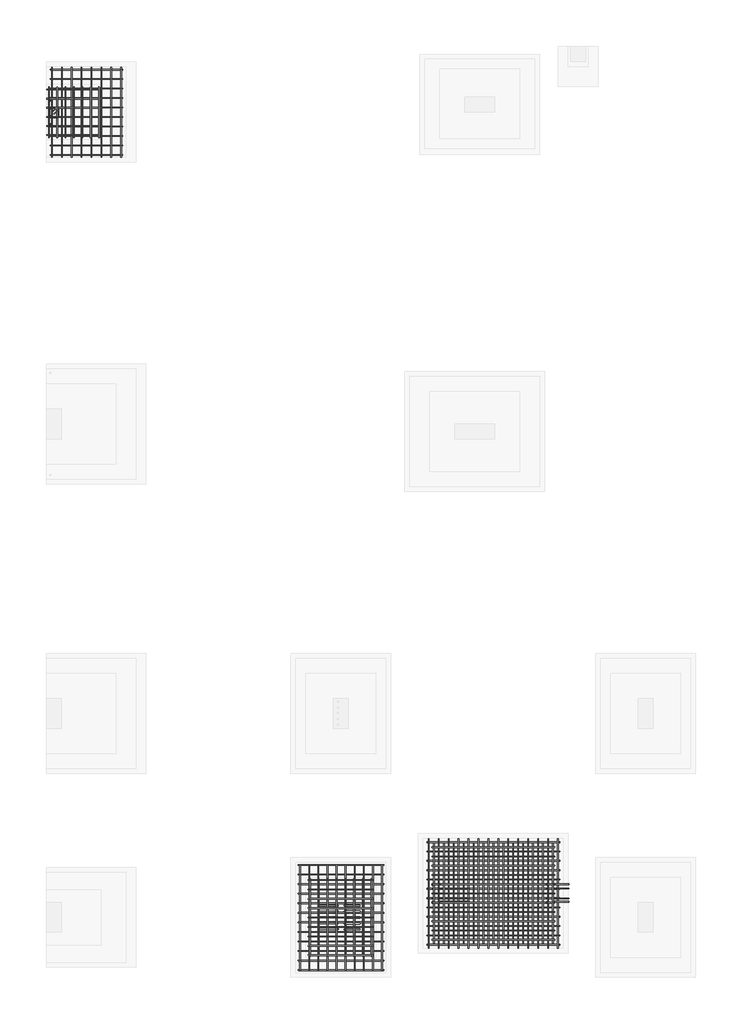
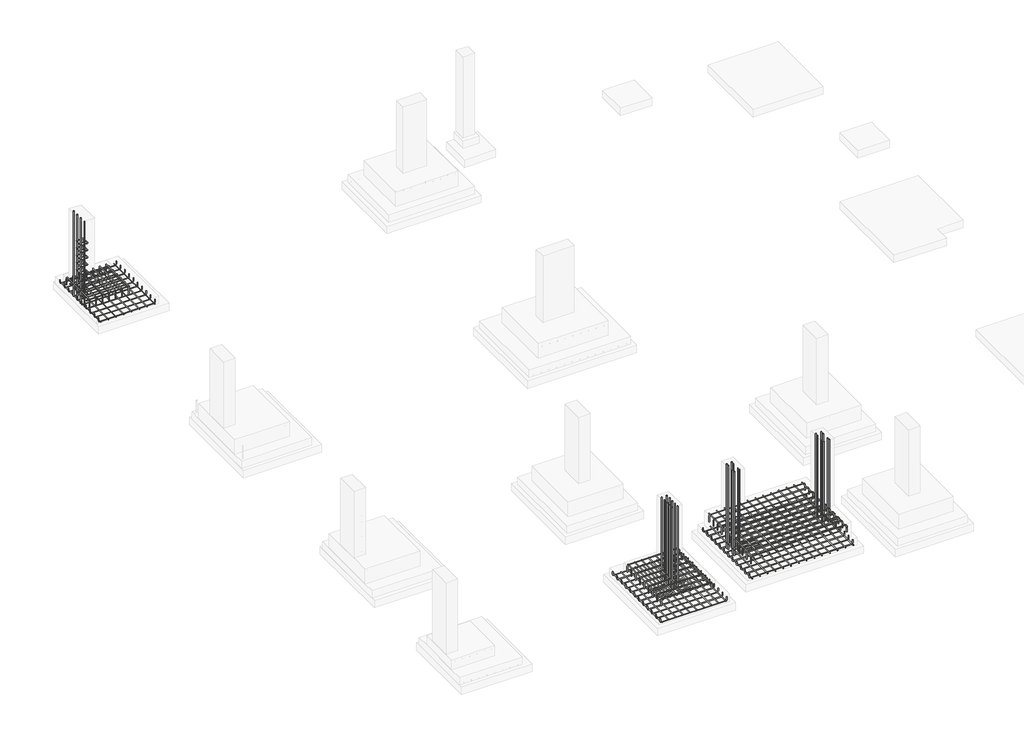
# One storey, part 3 of 6: 24 reinforcing bars.
"""IFC4 building model written with IfcOpenShell, lengths in millimetres."""

from ifc_helpers import new_model, si_unit, point, frame, origin, place, context, project, spatial, polyline, circle_curve, trimmed, segment, composite_curve, source, transform, mapped, element, save
from ifc_brep_helpers import swept_disk

model = new_model("IFC4")

# Units and contexts
model_context = context("Model", 3, world=origin())
ifc_project = project(units=[si_unit("LENGTHUNIT", "METRE", prefix="MILLI")], contexts=[model_context])

# Site, building, storey
site = spatial("IfcSite", under=ifc_project)
building = spatial("IfcBuilding", under=site)
storey = spatial("IfcBuildingStorey", under=building, Elevation=-1828.8)

# Reinforcing bars
placement = place(None, origin())
reinforcing_bar_shape = source(origin(), model_context, "Body", "SolidModel", [
    swept_disk(composite_curve([segment(polyline([(5667705.257242, -3596967.8875145, -1798.9561208), (5667705.257242, -3598584.2875145, -1798.9561208)]), True, "CONTINUOUS")], self_intersect=False), 6.0),
])
element("IfcReinforcingBar", 1, at=placement, inside=storey, context=model_context, shape_type="MappedRepresentation", body=[
    mapped(reinforcing_bar_shape, transform((0.0, 0.0, 0.0), x_axis=(1.0, 0.0, 0.0), y_axis=(0.0, 1.0, 0.0), z_axis=(0.0, 0.0, 1.0))),
    mapped(reinforcing_bar_shape, transform((-138.8763652, 0.0, 0.0), x_axis=(1.0, 0.0, 0.0), y_axis=(0.0, 1.0, 0.0), z_axis=(0.0, 0.0, 1.0))),
    mapped(reinforcing_bar_shape, transform((-277.7527305, 0.0, 0.0), x_axis=(1.0, 0.0, 0.0), y_axis=(0.0, 1.0, 0.0), z_axis=(0.0, 0.0, 1.0))),
    mapped(reinforcing_bar_shape, transform((-416.6290957, 0.0, 0.0), x_axis=(1.0, 0.0, 0.0), y_axis=(0.0, 1.0, 0.0), z_axis=(0.0, 0.0, 1.0))),
    mapped(reinforcing_bar_shape, transform((-555.5054609, 0.0, 0.0), x_axis=(1.0, 0.0, 0.0), y_axis=(0.0, 1.0, 0.0), z_axis=(0.0, 0.0, 1.0))),
    mapped(reinforcing_bar_shape, transform((-694.3818262, 0.0, 0.0), x_axis=(1.0, 0.0, 0.0), y_axis=(0.0, 1.0, 0.0), z_axis=(0.0, 0.0, 1.0))),
    mapped(reinforcing_bar_shape, transform((-833.2581914, 0.0, 0.0), x_axis=(1.0, 0.0, 0.0), y_axis=(0.0, 1.0, 0.0), z_axis=(0.0, 0.0, 1.0))),
    mapped(reinforcing_bar_shape, transform((-972.1345566, 0.0, 0.0), x_axis=(1.0, 0.0, 0.0), y_axis=(0.0, 1.0, 0.0), z_axis=(0.0, 0.0, 1.0))),
    mapped(reinforcing_bar_shape, transform((-1111.0109219, 0.0, 0.0), x_axis=(1.0, 0.0, 0.0), y_axis=(0.0, 1.0, 0.0), z_axis=(0.0, 0.0, 1.0))),
    mapped(reinforcing_bar_shape, transform((-1249.8872871, 0.0, 0.0), x_axis=(1.0, 0.0, 0.0), y_axis=(0.0, 1.0, 0.0), z_axis=(0.0, 0.0, 1.0))),
])
reinforcing_bar_2_shape = source(origin(), model_context, "Body", "SolidModel", [
    swept_disk(composite_curve([segment(polyline([(5666582.9165246, -3598349.6875145, -1653.2), (5666582.9165246, -3598349.6875145, -1539.2)]), True, "CONTINUOUS"), segment(trimmed(circle_curve(frame((5666612.9165246, -3598349.6875145, -1539.2), z_axis=(0.0, 1.0, 0.0), x_axis=(-30.0, 0.0, 0.0)), 30.0), [point((5666582.9165246, -3598349.6875145, -1539.2))], [point((5666612.9165246, -3598349.6875145, -1509.2))], True, "CARTESIAN"), True, "CONTINUOUS"), segment(polyline([(5666612.9165246, -3598349.6875145, -1509.2), (5667539.8524241, -3598349.6875145, -1509.2)]), True, "CONTINUOUS"), segment(trimmed(circle_curve(frame((5667539.8524241, -3598349.6875145, -1539.2), z_axis=(0.0, 1.0, 0.0), x_axis=(0.0, 0.0, 30.0)), 30.0), [point((5667539.8524241, -3598349.6875145, -1509.2))], [point((5667569.8524241, -3598349.6875145, -1539.2))], True, "CARTESIAN"), True, "CONTINUOUS"), segment(polyline([(5667569.8524241, -3598349.6875145, -1539.2), (5667569.8524241, -3598349.6875145, -1653.2)]), True, "CONTINUOUS")], self_intersect=False), 6.0),
])
element("IfcReinforcingBar", 2, at=placement, inside=storey, context=model_context, shape_type="MappedRepresentation", body=[
    mapped(reinforcing_bar_2_shape, transform((0.0, 0.0, 0.0), x_axis=(1.0, 0.0, 0.0), y_axis=(0.0, 1.0, 0.0), z_axis=(0.0, 0.0, 1.0))),
    mapped(reinforcing_bar_2_shape, transform((0.0, 143.4, 0.0), x_axis=(1.0, 0.0, 0.0), y_axis=(0.0, 1.0, 0.0), z_axis=(0.0, 0.0, 1.0))),
    mapped(reinforcing_bar_2_shape, transform((0.0, 286.8, 0.0), x_axis=(1.0, 0.0, 0.0), y_axis=(0.0, 1.0, 0.0), z_axis=(0.0, 0.0, 1.0))),
    mapped(reinforcing_bar_2_shape, transform((0.0, 430.2, 0.0), x_axis=(1.0, 0.0, 0.0), y_axis=(0.0, 1.0, 0.0), z_axis=(0.0, 0.0, 1.0))),
    mapped(reinforcing_bar_2_shape, transform((0.0, 573.6, 0.0), x_axis=(1.0, 0.0, 0.0), y_axis=(0.0, 1.0, 0.0), z_axis=(0.0, 0.0, 1.0))),
    mapped(reinforcing_bar_2_shape, transform((0.0, 717.0, 0.0), x_axis=(1.0, 0.0, 0.0), y_axis=(0.0, 1.0, 0.0), z_axis=(0.0, 0.0, 1.0))),
    mapped(reinforcing_bar_2_shape, transform((0.0, 860.4, 0.0), x_axis=(1.0, 0.0, 0.0), y_axis=(0.0, 1.0, 0.0), z_axis=(0.0, 0.0, 1.0))),
    mapped(reinforcing_bar_2_shape, transform((0.0, 1003.8, 0.0), x_axis=(1.0, 0.0, 0.0), y_axis=(0.0, 1.0, 0.0), z_axis=(0.0, 0.0, 1.0))),
    mapped(reinforcing_bar_2_shape, transform((0.0, 1147.2, 0.0), x_axis=(1.0, 0.0, 0.0), y_axis=(0.0, 1.0, 0.0), z_axis=(0.0, 0.0, 1.0))),
])
reinforcing_bar_3_shape = source(origin(), model_context, "Body", "SolidModel", [
    swept_disk(composite_curve([segment(polyline([(5666606.9072819, -3598369.1575222, -1522.1088801), (5666606.9072819, -3597181.5930968, -1522.1088801)]), True, "CONTINUOUS")], self_intersect=False), 6.0),
])
element("IfcReinforcingBar", 3, at=placement, inside=storey, context=model_context, shape_type="MappedRepresentation", body=[
    mapped(reinforcing_bar_3_shape, transform((0.0, 0.0, 0.0), x_axis=(1.0, 0.0, 0.0), y_axis=(0.0, 1.0, 0.0), z_axis=(0.0, 0.0, 1.0))),
    mapped(reinforcing_bar_3_shape, transform((133.9695725, 0.0, 0.0), x_axis=(1.0, 0.0, 0.0), y_axis=(0.0, 1.0, 0.0), z_axis=(0.0, 0.0, 1.0))),
    mapped(reinforcing_bar_3_shape, transform((267.939145, 0.0, 0.0), x_axis=(1.0, 0.0, 0.0), y_axis=(0.0, 1.0, 0.0), z_axis=(0.0, 0.0, 1.0))),
    mapped(reinforcing_bar_3_shape, transform((401.9087176, 0.0, 0.0), x_axis=(1.0, 0.0, 0.0), y_axis=(0.0, 1.0, 0.0), z_axis=(0.0, 0.0, 1.0))),
    mapped(reinforcing_bar_3_shape, transform((535.8782901, 0.0, 0.0), x_axis=(1.0, 0.0, 0.0), y_axis=(0.0, 1.0, 0.0), z_axis=(0.0, 0.0, 1.0))),
    mapped(reinforcing_bar_3_shape, transform((669.8478626, 0.0, 0.0), x_axis=(1.0, 0.0, 0.0), y_axis=(0.0, 1.0, 0.0), z_axis=(0.0, 0.0, 1.0))),
    mapped(reinforcing_bar_3_shape, transform((803.8174351, 0.0, 0.0), x_axis=(1.0, 0.0, 0.0), y_axis=(0.0, 1.0, 0.0), z_axis=(0.0, 0.0, 1.0))),
    mapped(reinforcing_bar_3_shape, transform((937.7870076, 0.0, 0.0), x_axis=(1.0, 0.0, 0.0), y_axis=(0.0, 1.0, 0.0), z_axis=(0.0, 0.0, 1.0))),
])
reinforcing_bar_4_shape = source(origin(), model_context, "Body", "SolidModel", [
    swept_disk(composite_curve([segment(polyline([(5662646.549334, -3584842.9113604, -1738.4709043), (5662646.549334, -3584842.9113604, -1793.4709043)]), True, "CONTINUOUS"), segment(trimmed(circle_curve(frame((5662671.549334, -3584842.9113604, -1793.4709043), z_axis=(0.0, -1.0, 0.0), x_axis=(-25.0, 0.0, 0.0)), 25.0), [point((5662646.549334, -3584842.9113604, -1793.4709043))], [point((5662671.549334, -3584842.9113604, -1818.4709043))], True, "CARTESIAN"), True, "CONTINUOUS"), segment(polyline([(5662671.549334, -3584842.9113604, -1818.4709043), (5663718.1378894, -3584842.9113604, -1818.4709043)]), True, "CONTINUOUS"), segment(trimmed(circle_curve(frame((5663718.1378894, -3584842.9113604, -1793.4709043), z_axis=(0.0, -1.0, 0.0), x_axis=(0.0, 0.0, -25.0)), 25.0), [point((5663718.1378894, -3584842.9113604, -1818.4709043))], [point((5663743.1378894, -3584842.9113604, -1793.4709043))], True, "CARTESIAN"), True, "CONTINUOUS"), segment(polyline([(5663743.1378894, -3584842.9113604, -1793.4709043), (5663743.1378894, -3584842.9113604, -1738.4709043)]), True, "CONTINUOUS")], self_intersect=False), 5.0),
])
element("IfcReinforcingBar", 4, at=placement, inside=storey, context=model_context, shape_type="MappedRepresentation", body=[
    mapped(reinforcing_bar_4_shape, transform((0.0, 0.0, 0.0), x_axis=(1.0, 0.0, 0.0), y_axis=(0.0, 1.0, 0.0), z_axis=(0.0, 0.0, 1.0))),
    mapped(reinforcing_bar_4_shape, transform((0.0, -144.6222222, 0.0), x_axis=(1.0, 0.0, 0.0), y_axis=(0.0, 1.0, 0.0), z_axis=(0.0, 0.0, 1.0))),
    mapped(reinforcing_bar_4_shape, transform((0.0, -289.2444444, 0.0), x_axis=(1.0, 0.0, 0.0), y_axis=(0.0, 1.0, 0.0), z_axis=(0.0, 0.0, 1.0))),
    mapped(reinforcing_bar_4_shape, transform((0.0, -433.8666667, 0.0), x_axis=(1.0, 0.0, 0.0), y_axis=(0.0, 1.0, 0.0), z_axis=(0.0, 0.0, 1.0))),
    mapped(reinforcing_bar_4_shape, transform((0.0, -578.4888889, 0.0), x_axis=(1.0, 0.0, 0.0), y_axis=(0.0, 1.0, 0.0), z_axis=(0.0, 0.0, 1.0))),
    mapped(reinforcing_bar_4_shape, transform((0.0, -723.1111111, 0.0), x_axis=(1.0, 0.0, 0.0), y_axis=(0.0, 1.0, 0.0), z_axis=(0.0, 0.0, 1.0))),
    mapped(reinforcing_bar_4_shape, transform((0.0, -867.7333333, 0.0), x_axis=(1.0, 0.0, 0.0), y_axis=(0.0, 1.0, 0.0), z_axis=(0.0, 0.0, 1.0))),
    mapped(reinforcing_bar_4_shape, transform((0.0, -1012.3555556, 0.0), x_axis=(1.0, 0.0, 0.0), y_axis=(0.0, 1.0, 0.0), z_axis=(0.0, 0.0, 1.0))),
    mapped(reinforcing_bar_4_shape, transform((0.0, -1156.9777778, 0.0), x_axis=(1.0, 0.0, 0.0), y_axis=(0.0, 1.0, 0.0), z_axis=(0.0, 0.0, 1.0))),
    mapped(reinforcing_bar_4_shape, transform((0.0, -1301.6, 0.0), x_axis=(1.0, 0.0, 0.0), y_axis=(0.0, 1.0, 0.0), z_axis=(0.0, 0.0, 1.0))),
])
reinforcing_bar_5_shape = source(origin(), model_context, "Body", "SolidModel", [
    swept_disk(composite_curve([segment(polyline([(5662668.193273, -3584807.9113604, -1807.7638193), (5662668.193273, -3586179.5113604, -1807.7638193)]), True, "CONTINUOUS")], self_intersect=False), 5.0),
])
element("IfcReinforcingBar", 5, at=placement, inside=storey, context=model_context, shape_type="MappedRepresentation", body=[
    mapped(reinforcing_bar_5_shape, transform((0.0, 0.0, 0.0), x_axis=(1.0, 0.0, 0.0), y_axis=(0.0, 1.0, 0.0), z_axis=(0.0, 0.0, 1.0))),
    mapped(reinforcing_bar_5_shape, transform((150.6667583, 0.0, 0.0), x_axis=(1.0, 0.0, 0.0), y_axis=(0.0, 1.0, 0.0), z_axis=(0.0, 0.0, 1.0))),
    mapped(reinforcing_bar_5_shape, transform((301.3335165, 0.0, 0.0), x_axis=(1.0, 0.0, 0.0), y_axis=(0.0, 1.0, 0.0), z_axis=(0.0, 0.0, 1.0))),
    mapped(reinforcing_bar_5_shape, transform((452.0002748, 0.0, 0.0), x_axis=(1.0, 0.0, 0.0), y_axis=(0.0, 1.0, 0.0), z_axis=(0.0, 0.0, 1.0))),
    mapped(reinforcing_bar_5_shape, transform((602.6670331, 0.0, 0.0), x_axis=(1.0, 0.0, 0.0), y_axis=(0.0, 1.0, 0.0), z_axis=(0.0, 0.0, 1.0))),
    mapped(reinforcing_bar_5_shape, transform((753.3337913, 0.0, 0.0), x_axis=(1.0, 0.0, 0.0), y_axis=(0.0, 1.0, 0.0), z_axis=(0.0, 0.0, 1.0))),
    mapped(reinforcing_bar_5_shape, transform((904.0005496, 0.0, 0.0), x_axis=(1.0, 0.0, 0.0), y_axis=(0.0, 1.0, 0.0), z_axis=(0.0, 0.0, 1.0))),
    mapped(reinforcing_bar_5_shape, transform((1054.6673079, 0.0, 0.0), x_axis=(1.0, 0.0, 0.0), y_axis=(0.0, 1.0, 0.0), z_axis=(0.0, 0.0, 1.0))),
])
reinforcing_bar_6_shape = source(origin(), model_context, "Body", "SolidModel", [
    swept_disk(composite_curve([segment(polyline([(5663387.7113073, -3585877.8113604, -1673.2), (5663387.7113073, -3585877.8113604, -1533.2)]), True, "CONTINUOUS"), segment(trimmed(circle_curve(frame((5663387.7113073, -3585852.8113604, -1533.2), z_axis=(-1.0, 0.0, 0.0), x_axis=(0.0, -25.0, 0.0)), 25.0), [point((5663387.7113073, -3585877.8113604, -1533.2))], [point((5663387.7113073, -3585852.8113604, -1508.2))], True, "CARTESIAN"), True, "CONTINUOUS"), segment(polyline([(5663387.7113073, -3585852.8113604, -1508.2), (5663387.7113073, -3585134.6113604, -1508.2)]), True, "CONTINUOUS"), segment(trimmed(circle_curve(frame((5663387.7113073, -3585134.6113604, -1533.2), z_axis=(-1.0, 0.0, 0.0), x_axis=(0.0, 0.0, 25.0)), 25.0), [point((5663387.7113073, -3585134.6113604, -1508.2))], [point((5663387.7113073, -3585109.6113604, -1533.2))], True, "CARTESIAN"), True, "CONTINUOUS"), segment(polyline([(5663387.7113073, -3585109.6113604, -1533.2), (5663387.7113073, -3585109.6113604, -1673.2)]), True, "CONTINUOUS")], self_intersect=False), 5.0),
])
element("IfcReinforcingBar", 6, at=placement, inside=storey, context=model_context, shape_type="MappedRepresentation", body=[
    mapped(reinforcing_bar_6_shape, transform((0.0, 0.0, 0.0), x_axis=(1.0, 0.0, 0.0), y_axis=(0.0, 1.0, 0.0), z_axis=(0.0, 0.0, 1.0))),
    mapped(reinforcing_bar_6_shape, transform((-128.0333333, 0.0, 0.0), x_axis=(1.0, 0.0, 0.0), y_axis=(0.0, 1.0, 0.0), z_axis=(0.0, 0.0, 1.0))),
    mapped(reinforcing_bar_6_shape, transform((-256.0666667, 0.0, 0.0), x_axis=(1.0, 0.0, 0.0), y_axis=(0.0, 1.0, 0.0), z_axis=(0.0, 0.0, 1.0))),
    mapped(reinforcing_bar_6_shape, transform((-384.1, 0.0, 0.0), x_axis=(1.0, 0.0, 0.0), y_axis=(0.0, 1.0, 0.0), z_axis=(0.0, 0.0, 1.0))),
    mapped(reinforcing_bar_6_shape, transform((-512.1333333, 0.0, 0.0), x_axis=(1.0, 0.0, 0.0), y_axis=(0.0, 1.0, 0.0), z_axis=(0.0, 0.0, 1.0))),
    mapped(reinforcing_bar_6_shape, transform((-640.1666667, 0.0, 0.0), x_axis=(1.0, 0.0, 0.0), y_axis=(0.0, 1.0, 0.0), z_axis=(0.0, 0.0, 1.0))),
    mapped(reinforcing_bar_6_shape, transform((-768.2, 0.0, 0.0), x_axis=(1.0, 0.0, 0.0), y_axis=(0.0, 1.0, 0.0), z_axis=(0.0, 0.0, 1.0))),
])
reinforcing_bar_7_shape = source(origin(), model_context, "Body", "SolidModel", [
    swept_disk(composite_curve([segment(polyline([(5663422.7113073, -3585840.4015215, -1540.036299), (5662584.5113073, -3585840.4015215, -1540.036299)]), True, "CONTINUOUS")], self_intersect=False), 5.0),
])
element("IfcReinforcingBar", 7, at=placement, inside=storey, context=model_context, shape_type="MappedRepresentation", body=[
    mapped(reinforcing_bar_7_shape, transform((0.0, 0.0, 0.0), x_axis=(1.0, 0.0, 0.0), y_axis=(0.0, 1.0, 0.0), z_axis=(0.0, 0.0, 1.0))),
    mapped(reinforcing_bar_7_shape, transform((0.0, 138.6844386, 0.0), x_axis=(1.0, 0.0, 0.0), y_axis=(0.0, 1.0, 0.0), z_axis=(0.0, 0.0, 1.0))),
    mapped(reinforcing_bar_7_shape, transform((0.0, 277.3688772, 0.0), x_axis=(1.0, 0.0, 0.0), y_axis=(0.0, 1.0, 0.0), z_axis=(0.0, 0.0, 1.0))),
    mapped(reinforcing_bar_7_shape, transform((0.0, 416.0533158, 0.0), x_axis=(1.0, 0.0, 0.0), y_axis=(0.0, 1.0, 0.0), z_axis=(0.0, 0.0, 1.0))),
    mapped(reinforcing_bar_7_shape, transform((0.0, 554.7377544, 0.0), x_axis=(1.0, 0.0, 0.0), y_axis=(0.0, 1.0, 0.0), z_axis=(0.0, 0.0, 1.0))),
    mapped(reinforcing_bar_7_shape, transform((0.0, 693.422193, 0.0), x_axis=(1.0, 0.0, 0.0), y_axis=(0.0, 1.0, 0.0), z_axis=(0.0, 0.0, 1.0))),
])
reinforcing_bar_8_shape = source(origin(), model_context, "Body", "SolidModel", [
    swept_disk(composite_curve([segment(polyline([(5668393.6165246, -3596625.5875145, -1733.8446259), (5668393.6165246, -3596625.5875145, -1782.8446259)]), True, "CONTINUOUS"), segment(trimmed(circle_curve(frame((5668423.6165246, -3596625.5875145, -1782.8446259), z_axis=(0.0, -1.0, 0.0), x_axis=(-30.0, 0.0, 0.0)), 30.0), [point((5668393.6165246, -3596625.5875145, -1782.8446259))], [point((5668423.6165246, -3596625.5875145, -1812.8446259))], True, "CARTESIAN"), True, "CONTINUOUS"), segment(polyline([(5668423.6165246, -3596625.5875145, -1812.8446259), (5670385.2165246, -3596625.5875145, -1812.8446259)]), True, "CONTINUOUS"), segment(trimmed(circle_curve(frame((5670385.2165246, -3596625.5875145, -1782.8446259), z_axis=(0.0, -1.0, 0.0), x_axis=(0.0, 0.0, -30.0)), 30.0), [point((5670385.2165246, -3596625.5875145, -1812.8446259))], [point((5670415.2165246, -3596625.5875145, -1782.8446259))], True, "CARTESIAN"), True, "CONTINUOUS"), segment(polyline([(5670415.2165246, -3596625.5875145, -1782.8446259), (5670415.2165246, -3596625.5875145, -1733.8446259)]), True, "CONTINUOUS")], self_intersect=False), 6.0),
])
element("IfcReinforcingBar", 8, at=placement, inside=storey, context=model_context, shape_type="MappedRepresentation", body=[
    mapped(reinforcing_bar_8_shape, transform((0.0, 0.0, 0.0), x_axis=(1.0, 0.0, 0.0), y_axis=(0.0, 1.0, 0.0), z_axis=(0.0, 0.0, 1.0))),
    mapped(reinforcing_bar_8_shape, transform((0.0, -142.2181818, 0.0), x_axis=(1.0, 0.0, 0.0), y_axis=(0.0, 1.0, 0.0), z_axis=(0.0, 0.0, 1.0))),
    mapped(reinforcing_bar_8_shape, transform((0.0, -284.4363636, 0.0), x_axis=(1.0, 0.0, 0.0), y_axis=(0.0, 1.0, 0.0), z_axis=(0.0, 0.0, 1.0))),
    mapped(reinforcing_bar_8_shape, transform((0.0, -426.6545455, 0.0), x_axis=(1.0, 0.0, 0.0), y_axis=(0.0, 1.0, 0.0), z_axis=(0.0, 0.0, 1.0))),
    mapped(reinforcing_bar_8_shape, transform((0.0, -568.8727273, 0.0), x_axis=(1.0, 0.0, 0.0), y_axis=(0.0, 1.0, 0.0), z_axis=(0.0, 0.0, 1.0))),
    mapped(reinforcing_bar_8_shape, transform((0.0, -711.0909091, 0.0), x_axis=(1.0, 0.0, 0.0), y_axis=(0.0, 1.0, 0.0), z_axis=(0.0, 0.0, 1.0))),
    mapped(reinforcing_bar_8_shape, transform((0.0, -853.3090909, 0.0), x_axis=(1.0, 0.0, 0.0), y_axis=(0.0, 1.0, 0.0), z_axis=(0.0, 0.0, 1.0))),
    mapped(reinforcing_bar_8_shape, transform((0.0, -995.5272727, 0.0), x_axis=(1.0, 0.0, 0.0), y_axis=(0.0, 1.0, 0.0), z_axis=(0.0, 0.0, 1.0))),
    mapped(reinforcing_bar_8_shape, transform((0.0, -1137.7454545, 0.0), x_axis=(1.0, 0.0, 0.0), y_axis=(0.0, 1.0, 0.0), z_axis=(0.0, 0.0, 1.0))),
    mapped(reinforcing_bar_8_shape, transform((0.0, -1279.9636364, 0.0), x_axis=(1.0, 0.0, 0.0), y_axis=(0.0, 1.0, 0.0), z_axis=(0.0, 0.0, 1.0))),
    mapped(reinforcing_bar_8_shape, transform((0.0, -1422.1818182, 0.0), x_axis=(1.0, 0.0, 0.0), y_axis=(0.0, 1.0, 0.0), z_axis=(0.0, 0.0, 1.0))),
    mapped(reinforcing_bar_8_shape, transform((0.0, -1564.4, 0.0), x_axis=(1.0, 0.0, 0.0), y_axis=(0.0, 1.0, 0.0), z_axis=(0.0, 0.0, 1.0))),
])
reinforcing_bar_9_shape = source(origin(), model_context, "Body", "SolidModel", [
    swept_disk(composite_curve([segment(polyline([(5670339.0165246, -3596701.7875145, -1583.6477635), (5670339.0165246, -3596701.7875145, -1469.6477635)]), True, "CONTINUOUS"), segment(trimmed(circle_curve(frame((5670309.0165246, -3596701.7875145, -1469.6477635), z_axis=(0.0, -1.0, 0.0), x_axis=(30.0, 0.0, 0.0)), 30.0), [point((5670339.0165246, -3596701.7875145, -1469.6477635))], [point((5670309.0165246, -3596701.7875145, -1439.6477635))], True, "CARTESIAN"), True, "CONTINUOUS"), segment(polyline([(5670309.0165246, -3596701.7875145, -1439.6477635), (5668499.8165246, -3596701.7875145, -1439.6477635)]), True, "CONTINUOUS"), segment(trimmed(circle_curve(frame((5668499.8165246, -3596701.7875145, -1469.6477635), z_axis=(0.0, -1.0, 0.0), x_axis=(0.0, 0.0, 30.0)), 30.0), [point((5668499.8165246, -3596701.7875145, -1439.6477635))], [point((5668469.8165246, -3596701.7875145, -1469.6477635))], True, "CARTESIAN"), True, "CONTINUOUS"), segment(polyline([(5668469.8165246, -3596701.7875145, -1469.6477635), (5668469.8165246, -3596701.7875145, -1583.6477635)]), True, "CONTINUOUS")], self_intersect=False), 6.0),
])
element("IfcReinforcingBar", 9, at=placement, inside=storey, context=model_context, shape_type="MappedRepresentation", body=[
    mapped(reinforcing_bar_9_shape, transform((0.0, 0.0, 0.0), x_axis=(1.0, 0.0, 0.0), y_axis=(0.0, 1.0, 0.0), z_axis=(0.0, 0.0, 1.0))),
    mapped(reinforcing_bar_9_shape, transform((0.0, -141.2, 0.0), x_axis=(1.0, 0.0, 0.0), y_axis=(0.0, 1.0, 0.0), z_axis=(0.0, 0.0, 1.0))),
    mapped(reinforcing_bar_9_shape, transform((0.0, -282.4, 0.0), x_axis=(1.0, 0.0, 0.0), y_axis=(0.0, 1.0, 0.0), z_axis=(0.0, 0.0, 1.0))),
    mapped(reinforcing_bar_9_shape, transform((0.0, -423.6, 0.0), x_axis=(1.0, 0.0, 0.0), y_axis=(0.0, 1.0, 0.0), z_axis=(0.0, 0.0, 1.0))),
    mapped(reinforcing_bar_9_shape, transform((0.0, -564.8, 0.0), x_axis=(1.0, 0.0, 0.0), y_axis=(0.0, 1.0, 0.0), z_axis=(0.0, 0.0, 1.0))),
    mapped(reinforcing_bar_9_shape, transform((0.0, -706.0, 0.0), x_axis=(1.0, 0.0, 0.0), y_axis=(0.0, 1.0, 0.0), z_axis=(0.0, 0.0, 1.0))),
    mapped(reinforcing_bar_9_shape, transform((0.0, -847.2, 0.0), x_axis=(1.0, 0.0, 0.0), y_axis=(0.0, 1.0, 0.0), z_axis=(0.0, 0.0, 1.0))),
    mapped(reinforcing_bar_9_shape, transform((0.0, -988.4, 0.0), x_axis=(1.0, 0.0, 0.0), y_axis=(0.0, 1.0, 0.0), z_axis=(0.0, 0.0, 1.0))),
    mapped(reinforcing_bar_9_shape, transform((0.0, -1129.6, 0.0), x_axis=(1.0, 0.0, 0.0), y_axis=(0.0, 1.0, 0.0), z_axis=(0.0, 0.0, 1.0))),
    mapped(reinforcing_bar_9_shape, transform((0.0, -1270.8, 0.0), x_axis=(1.0, 0.0, 0.0), y_axis=(0.0, 1.0, 0.0), z_axis=(0.0, 0.0, 1.0))),
    mapped(reinforcing_bar_9_shape, transform((0.0, -1412.0, 0.0), x_axis=(1.0, 0.0, 0.0), y_axis=(0.0, 1.0, 0.0), z_axis=(0.0, 0.0, 1.0))),
])
reinforcing_bar_10_shape = source(origin(), model_context, "Body", "SolidModel", [
    swept_disk(composite_curve([segment(polyline([(5668418.2145873, -3596569.5875145, -1800.1641527), (5668418.2145873, -3598245.9875145, -1800.1641527)]), True, "CONTINUOUS")], self_intersect=False), 6.0),
])
element("IfcReinforcingBar", 10, at=placement, inside=storey, context=model_context, shape_type="MappedRepresentation", body=[
    mapped(reinforcing_bar_10_shape, transform((0.0, 0.0, 0.0), x_axis=(1.0, 0.0, 0.0), y_axis=(0.0, 1.0, 0.0), z_axis=(0.0, 0.0, 1.0))),
    mapped(reinforcing_bar_10_shape, transform((151.7473845, 0.0, 0.0), x_axis=(1.0, 0.0, 0.0), y_axis=(0.0, 1.0, 0.0), z_axis=(0.0, 0.0, 1.0))),
    mapped(reinforcing_bar_10_shape, transform((303.4947691, 0.0, 0.0), x_axis=(1.0, 0.0, 0.0), y_axis=(0.0, 1.0, 0.0), z_axis=(0.0, 0.0, 1.0))),
    mapped(reinforcing_bar_10_shape, transform((455.2421536, 0.0, 0.0), x_axis=(1.0, 0.0, 0.0), y_axis=(0.0, 1.0, 0.0), z_axis=(0.0, 0.0, 1.0))),
    mapped(reinforcing_bar_10_shape, transform((606.9895382, 0.0, 0.0), x_axis=(1.0, 0.0, 0.0), y_axis=(0.0, 1.0, 0.0), z_axis=(0.0, 0.0, 1.0))),
    mapped(reinforcing_bar_10_shape, transform((758.7369227, 0.0, 0.0), x_axis=(1.0, 0.0, 0.0), y_axis=(0.0, 1.0, 0.0), z_axis=(0.0, 0.0, 1.0))),
    mapped(reinforcing_bar_10_shape, transform((910.4843073, 0.0, 0.0), x_axis=(1.0, 0.0, 0.0), y_axis=(0.0, 1.0, 0.0), z_axis=(0.0, 0.0, 1.0))),
    mapped(reinforcing_bar_10_shape, transform((1062.2316918, 0.0, 0.0), x_axis=(1.0, 0.0, 0.0), y_axis=(0.0, 1.0, 0.0), z_axis=(0.0, 0.0, 1.0))),
    mapped(reinforcing_bar_10_shape, transform((1213.9790763, 0.0, 0.0), x_axis=(1.0, 0.0, 0.0), y_axis=(0.0, 1.0, 0.0), z_axis=(0.0, 0.0, 1.0))),
    mapped(reinforcing_bar_10_shape, transform((1365.7264609, 0.0, 0.0), x_axis=(1.0, 0.0, 0.0), y_axis=(0.0, 1.0, 0.0), z_axis=(0.0, 0.0, 1.0))),
    mapped(reinforcing_bar_10_shape, transform((1517.4738454, 0.0, 0.0), x_axis=(1.0, 0.0, 0.0), y_axis=(0.0, 1.0, 0.0), z_axis=(0.0, 0.0, 1.0))),
    mapped(reinforcing_bar_10_shape, transform((1669.22123, 0.0, 0.0), x_axis=(1.0, 0.0, 0.0), y_axis=(0.0, 1.0, 0.0), z_axis=(0.0, 0.0, 1.0))),
    mapped(reinforcing_bar_10_shape, transform((1820.9686145, 0.0, 0.0), x_axis=(1.0, 0.0, 0.0), y_axis=(0.0, 1.0, 0.0), z_axis=(0.0, 0.0, 1.0))),
    mapped(reinforcing_bar_10_shape, transform((1972.715999, 0.0, 0.0), x_axis=(1.0, 0.0, 0.0), y_axis=(0.0, 1.0, 0.0), z_axis=(0.0, 0.0, 1.0))),
])
reinforcing_bar_11_shape = source(origin(), model_context, "Body", "SolidModel", [
    swept_disk(composite_curve([segment(polyline([(5670312.3233321, -3596645.7875145, -1451.7143428), (5670312.3233321, -3598169.7875145, -1451.7143428)]), True, "CONTINUOUS")], self_intersect=False), 6.0),
])
element("IfcReinforcingBar", 11, at=placement, inside=storey, context=model_context, shape_type="MappedRepresentation", body=[
    mapped(reinforcing_bar_11_shape, transform((0.0, 0.0, 0.0), x_axis=(1.0, 0.0, 0.0), y_axis=(0.0, 1.0, 0.0), z_axis=(0.0, 0.0, 1.0))),
    mapped(reinforcing_bar_11_shape, transform((-151.1594094, 0.0, 0.0), x_axis=(1.0, 0.0, 0.0), y_axis=(0.0, 1.0, 0.0), z_axis=(0.0, 0.0, 1.0))),
    mapped(reinforcing_bar_11_shape, transform((-302.3188187, 0.0, 0.0), x_axis=(1.0, 0.0, 0.0), y_axis=(0.0, 1.0, 0.0), z_axis=(0.0, 0.0, 1.0))),
    mapped(reinforcing_bar_11_shape, transform((-453.4782281, 0.0, 0.0), x_axis=(1.0, 0.0, 0.0), y_axis=(0.0, 1.0, 0.0), z_axis=(0.0, 0.0, 1.0))),
    mapped(reinforcing_bar_11_shape, transform((-604.6376374, 0.0, 0.0), x_axis=(1.0, 0.0, 0.0), y_axis=(0.0, 1.0, 0.0), z_axis=(0.0, 0.0, 1.0))),
    mapped(reinforcing_bar_11_shape, transform((-755.7970468, 0.0, 0.0), x_axis=(1.0, 0.0, 0.0), y_axis=(0.0, 1.0, 0.0), z_axis=(0.0, 0.0, 1.0))),
    mapped(reinforcing_bar_11_shape, transform((-906.9564561, 0.0, 0.0), x_axis=(1.0, 0.0, 0.0), y_axis=(0.0, 1.0, 0.0), z_axis=(0.0, 0.0, 1.0))),
    mapped(reinforcing_bar_11_shape, transform((-1058.1158655, 0.0, 0.0), x_axis=(1.0, 0.0, 0.0), y_axis=(0.0, 1.0, 0.0), z_axis=(0.0, 0.0, 1.0))),
    mapped(reinforcing_bar_11_shape, transform((-1209.2752749, 0.0, 0.0), x_axis=(1.0, 0.0, 0.0), y_axis=(0.0, 1.0, 0.0), z_axis=(0.0, 0.0, 1.0))),
    mapped(reinforcing_bar_11_shape, transform((-1360.4346842, 0.0, 0.0), x_axis=(1.0, 0.0, 0.0), y_axis=(0.0, 1.0, 0.0), z_axis=(0.0, 0.0, 1.0))),
    mapped(reinforcing_bar_11_shape, transform((-1511.5940936, 0.0, 0.0), x_axis=(1.0, 0.0, 0.0), y_axis=(0.0, 1.0, 0.0), z_axis=(0.0, 0.0, 1.0))),
    mapped(reinforcing_bar_11_shape, transform((-1662.7535029, 0.0, 0.0), x_axis=(1.0, 0.0, 0.0), y_axis=(0.0, 1.0, 0.0), z_axis=(0.0, 0.0, 1.0))),
    mapped(reinforcing_bar_11_shape, transform((-1813.9129123, 0.0, 0.0), x_axis=(1.0, 0.0, 0.0), y_axis=(0.0, 1.0, 0.0), z_axis=(0.0, 0.0, 1.0))),
])
reinforcing_bar_12_shape = source(origin(), model_context, "Body", "SolidModel", [
    swept_disk(composite_curve([segment(polyline([(5666430.5165246, -3596973.8875145, -1732.7232055), (5666430.5165246, -3596973.8875145, -1781.7232055)]), True, "CONTINUOUS"), segment(trimmed(circle_curve(frame((5666460.5165246, -3596973.8875145, -1781.7232055), z_axis=(0.0, -1.0, 0.0), x_axis=(-30.0, 0.0, 0.0)), 30.0), [point((5666430.5165246, -3596973.8875145, -1781.7232055))], [point((5666460.5165246, -3596973.8875145, -1811.7232055))], True, "CARTESIAN"), True, "CONTINUOUS"), segment(polyline([(5666460.5165246, -3596973.8875145, -1811.7232055), (5667700.1165246, -3596973.8875145, -1811.7232055)]), True, "CONTINUOUS"), segment(trimmed(circle_curve(frame((5667700.1165246, -3596973.8875145, -1781.7232055), z_axis=(0.0, -1.0, 0.0), x_axis=(0.0, 0.0, -30.0)), 30.0), [point((5667700.1165246, -3596973.8875145, -1811.7232055))], [point((5667730.1165246, -3596973.8875145, -1781.7232055))], True, "CARTESIAN"), True, "CONTINUOUS"), segment(polyline([(5667730.1165246, -3596973.8875145, -1781.7232055), (5667730.1165246, -3596973.8875145, -1732.7232055)]), True, "CONTINUOUS")], self_intersect=False), 6.0),
])
element("IfcReinforcingBar", 12, at=placement, inside=storey, context=model_context, shape_type="MappedRepresentation", body=[
    mapped(reinforcing_bar_12_shape, transform((0.0, 0.0, 0.0), x_axis=(1.0, 0.0, 0.0), y_axis=(0.0, 1.0, 0.0), z_axis=(0.0, 0.0, 1.0))),
    mapped(reinforcing_bar_12_shape, transform((0.0, -145.8545455, 0.0), x_axis=(1.0, 0.0, 0.0), y_axis=(0.0, 1.0, 0.0), z_axis=(0.0, 0.0, 1.0))),
    mapped(reinforcing_bar_12_shape, transform((0.0, -291.7090909, 0.0), x_axis=(1.0, 0.0, 0.0), y_axis=(0.0, 1.0, 0.0), z_axis=(0.0, 0.0, 1.0))),
    mapped(reinforcing_bar_12_shape, transform((0.0, -437.5636364, 0.0), x_axis=(1.0, 0.0, 0.0), y_axis=(0.0, 1.0, 0.0), z_axis=(0.0, 0.0, 1.0))),
    mapped(reinforcing_bar_12_shape, transform((0.0, -583.4181818, 0.0), x_axis=(1.0, 0.0, 0.0), y_axis=(0.0, 1.0, 0.0), z_axis=(0.0, 0.0, 1.0))),
    mapped(reinforcing_bar_12_shape, transform((0.0, -729.2727273, 0.0), x_axis=(1.0, 0.0, 0.0), y_axis=(0.0, 1.0, 0.0), z_axis=(0.0, 0.0, 1.0))),
    mapped(reinforcing_bar_12_shape, transform((0.0, -875.1272727, 0.0), x_axis=(1.0, 0.0, 0.0), y_axis=(0.0, 1.0, 0.0), z_axis=(0.0, 0.0, 1.0))),
    mapped(reinforcing_bar_12_shape, transform((0.0, -1020.9818182, 0.0), x_axis=(1.0, 0.0, 0.0), y_axis=(0.0, 1.0, 0.0), z_axis=(0.0, 0.0, 1.0))),
    mapped(reinforcing_bar_12_shape, transform((0.0, -1166.8363636, 0.0), x_axis=(1.0, 0.0, 0.0), y_axis=(0.0, 1.0, 0.0), z_axis=(0.0, 0.0, 1.0))),
    mapped(reinforcing_bar_12_shape, transform((0.0, -1312.6909091, 0.0), x_axis=(1.0, 0.0, 0.0), y_axis=(0.0, 1.0, 0.0), z_axis=(0.0, 0.0, 1.0))),
    mapped(reinforcing_bar_12_shape, transform((0.0, -1458.5454545, 0.0), x_axis=(1.0, 0.0, 0.0), y_axis=(0.0, 1.0, 0.0), z_axis=(0.0, 0.0, 1.0))),
    mapped(reinforcing_bar_12_shape, transform((0.0, -1604.4, 0.0), x_axis=(1.0, 0.0, 0.0), y_axis=(0.0, 1.0, 0.0), z_axis=(0.0, 0.0, 1.0))),
])
reinforcing_bar_13_shape = source(origin(), model_context, "Body", "SolidModel", [
    swept_disk(composite_curve([segment(polyline([(5662641.6613073, -3585313.9151054, -30.0), (5662641.6613073, -3585313.9151054, -1788.95)]), True, "CONTINUOUS")], self_intersect=False), 8.0),
])
element("IfcReinforcingBar", 13, at=placement, inside=storey, context=model_context, shape_type="MappedRepresentation", body=[
    mapped(reinforcing_bar_13_shape, transform((0.0, 0.0, 0.0), x_axis=(1.0, 0.0, 0.0), y_axis=(0.0, 1.0, 0.0), z_axis=(0.0, 0.0, 1.0))),
    mapped(reinforcing_bar_13_shape, transform((0.0, -120.1712362, 0.0), x_axis=(1.0, 0.0, 0.0), y_axis=(0.0, 1.0, 0.0), z_axis=(0.0, 0.0, 1.0))),
    mapped(reinforcing_bar_13_shape, transform((0.0, -240.3424723, 0.0), x_axis=(1.0, 0.0, 0.0), y_axis=(0.0, 1.0, 0.0), z_axis=(0.0, 0.0, 1.0))),
    mapped(reinforcing_bar_13_shape, transform((0.0, -360.5137085, 0.0), x_axis=(1.0, 0.0, 0.0), y_axis=(0.0, 1.0, 0.0), z_axis=(0.0, 0.0, 1.0))),
])
reinforcing_bar_14_shape = source(origin(), model_context, "Body", "SolidModel", [
    swept_disk(composite_curve([segment(polyline([(5662671.0775419, -3585489.6983058, -584.2), (5662735.4242589, -3585425.3515887, -584.2)]), True, "CONTINUOUS"), segment(trimmed(circle_curve(frame((5662749.5663946, -3585439.4937244, -584.2), z_axis=(0.0, 0.0, -1.0), x_axis=(-14.142135700210929, 14.142135700210929, 0.0)), 20.0), [point((5662735.4242589, -3585425.3515887, -584.2))], [point((5662769.5663946, -3585439.4937244, -584.2))], True, "CARTESIAN"), True, "CONTINUOUS"), segment(polyline([(5662769.5663946, -3585439.4937244, -584.2), (5662769.5663946, -3585553.9688111, -584.2)]), True, "CONTINUOUS"), segment(trimmed(circle_curve(frame((5662749.5663946, -3585553.9688111, -584.2), z_axis=(0.0, 0.0, -1.0), x_axis=(20.0, 0.0, 0.0)), 20.0), [point((5662769.5663946, -3585553.9688111, -584.2))], [point((5662749.5663946, -3585573.9688111, -584.2))], True, "CARTESIAN"), True, "CONTINUOUS"), segment(polyline([(5662749.5663946, -3585573.9688111, -584.2), (5662647.4163992, -3585573.9688111, -584.2)]), True, "CONTINUOUS"), segment(trimmed(circle_curve(frame((5662647.4163992, -3585553.9955776, -583.1656205), z_axis=(0.0, 0.05171897678513386, -0.9986616781674859), x_axis=(0.0, -19.97323350002989, -1.0343795)), 20.0), [point((5662647.4163992, -3585573.9688111, -584.2))], [point((5662627.4163992, -3585553.9955776, -583.1656205))], True, "CARTESIAN"), True, "CONTINUOUS"), segment(polyline([(5662627.4163992, -3585553.9955776, -583.1656205), (5662627.4163992, -3585439.4669579, -577.2343795)]), True, "CONTINUOUS"), segment(trimmed(circle_curve(frame((5662647.4163992, -3585439.4669579, -577.2343795), z_axis=(0.0, 0.05171897678513386, -0.9986616781674859), x_axis=(-20.0, 0.0, 0.0)), 20.0), [point((5662627.4163992, -3585439.4669579, -577.2343795))], [point((5662647.4163992, -3585419.4937244, -576.2))], True, "CARTESIAN"), True, "CONTINUOUS"), segment(polyline([(5662647.4163992, -3585419.4937244, -576.2), (5662749.5663946, -3585419.4937244, -576.2)]), True, "CONTINUOUS"), segment(trimmed(circle_curve(frame((5662749.5663946, -3585439.4937244, -576.2), z_axis=(0.0, 0.0, -1.0), x_axis=(0.0, 20.0, 0.0)), 20.0), [point((5662749.5663946, -3585419.4937244, -576.2))], [point((5662763.7085302, -3585453.63586, -576.2))], True, "CARTESIAN"), True, "CONTINUOUS"), segment(polyline([(5662763.7085302, -3585453.63586, -576.2), (5662699.3618131, -3585517.9825771, -576.2)]), True, "CONTINUOUS")], self_intersect=False), 4.0),
])
element("IfcReinforcingBar", 14, at=placement, inside=storey, context=model_context, shape_type="MappedRepresentation", body=[
    mapped(reinforcing_bar_14_shape, transform((0.0, 0.0, 0.0), x_axis=(1.0, 0.0, 0.0), y_axis=(0.0, 1.0, 0.0), z_axis=(0.0, 0.0, 1.0))),
    mapped(reinforcing_bar_14_shape, transform((0.0, 0.0, -149.5941627), x_axis=(1.0, 0.0, 0.0), y_axis=(0.0, 1.0, 0.0), z_axis=(0.0, 0.0, 1.0))),
    mapped(reinforcing_bar_14_shape, transform((0.0, 0.0, -299.1883255), x_axis=(1.0, 0.0, 0.0), y_axis=(0.0, 1.0, 0.0), z_axis=(0.0, 0.0, 1.0))),
    mapped(reinforcing_bar_14_shape, transform((0.0, 0.0, -448.7824882), x_axis=(1.0, 0.0, 0.0), y_axis=(0.0, 1.0, 0.0), z_axis=(0.0, 0.0, 1.0))),
    mapped(reinforcing_bar_14_shape, transform((0.0, 0.0, -598.3766509), x_axis=(1.0, 0.0, 0.0), y_axis=(0.0, 1.0, 0.0), z_axis=(0.0, 0.0, 1.0))),
    mapped(reinforcing_bar_14_shape, transform((0.0, 0.0, -747.9708137), x_axis=(1.0, 0.0, 0.0), y_axis=(0.0, 1.0, 0.0), z_axis=(0.0, 0.0, 1.0))),
    mapped(reinforcing_bar_14_shape, transform((0.0, 0.0, -897.5649764), x_axis=(1.0, 0.0, 0.0), y_axis=(0.0, 1.0, 0.0), z_axis=(0.0, 0.0, 1.0))),
    mapped(reinforcing_bar_14_shape, transform((0.0, 0.0, -1047.1591391), x_axis=(1.0, 0.0, 0.0), y_axis=(0.0, 1.0, 0.0), z_axis=(0.0, 0.0, 1.0))),
])
reinforcing_bar_15_shape = source(origin(), model_context, "Body", "SolidModel", [
    swept_disk(composite_curve([segment(polyline([(5667130.5836861, -3597591.8975754, -30.0), (5667130.5836861, -3597591.8975754, -1746.25)]), True, "CONTINUOUS"), segment(trimmed(circle_curve(frame((5667170.5836861, -3597591.8975754, -1746.25), z_axis=(0.0, -1.0, 0.0), x_axis=(-40.0, 0.0, 0.0)), 40.0), [point((5667130.5836861, -3597591.8975754, -1746.25))], [point((5667170.5836861, -3597591.8975754, -1786.25))], True, "CARTESIAN"), True, "CONTINUOUS"), segment(polyline([(5667170.5836861, -3597591.8975754, -1786.25), (5667372.4702744, -3597591.8975754, -1786.25)]), True, "CONTINUOUS")], self_intersect=False), 8.0),
])
element("IfcReinforcingBar", 15, at=placement, inside=storey, context=model_context, shape_type="MappedRepresentation", body=[
    mapped(reinforcing_bar_15_shape, transform((0.0, 0.0, 0.0), x_axis=(1.0, 0.0, 0.0), y_axis=(0.0, 1.0, 0.0), z_axis=(0.0, 0.0, 1.0))),
    mapped(reinforcing_bar_15_shape, transform((0.0, -91.3, 0.0), x_axis=(1.0, 0.0, 0.0), y_axis=(0.0, 1.0, 0.0), z_axis=(0.0, 0.0, 1.0))),
    mapped(reinforcing_bar_15_shape, transform((0.0, -182.6, 0.0), x_axis=(1.0, 0.0, 0.0), y_axis=(0.0, 1.0, 0.0), z_axis=(0.0, 0.0, 1.0))),
    mapped(reinforcing_bar_15_shape, transform((0.0, -273.9, 0.0), x_axis=(1.0, 0.0, 0.0), y_axis=(0.0, 1.0, 0.0), z_axis=(0.0, 0.0, 1.0))),
    mapped(reinforcing_bar_15_shape, transform((0.0, -365.2, 0.0), x_axis=(1.0, 0.0, 0.0), y_axis=(0.0, 1.0, 0.0), z_axis=(0.0, 0.0, 1.0))),
])
reinforcing_bar_16_shape = source(origin(), model_context, "Body", "SolidModel", [
    swept_disk(composite_curve([segment(polyline([(5667030.5419947, -3597594.7530253, -30.0), (5667030.5419947, -3597594.7530253, -1745.1487332)]), True, "CONTINUOUS"), segment(trimmed(circle_curve(frame((5666990.5419947, -3597594.7530253, -1745.1487332), z_axis=(0.0, 1.0, 0.0), x_axis=(40.0, 0.0, 0.0)), 40.0), [point((5667030.5419947, -3597594.7530253, -1745.1487332))], [point((5666990.5419947, -3597594.7530253, -1785.1487332))], True, "CARTESIAN"), True, "CONTINUOUS"), segment(polyline([(5666990.5419947, -3597594.7530253, -1785.1487332), (5666725.3079881, -3597594.7530253, -1785.1487332)]), True, "CONTINUOUS")], self_intersect=False), 8.0),
])
element("IfcReinforcingBar", 16, at=placement, inside=storey, context=model_context, shape_type="MappedRepresentation", body=[
    mapped(reinforcing_bar_16_shape, transform((0.0, 0.0, 0.0), x_axis=(1.0, 0.0, 0.0), y_axis=(0.0, 1.0, 0.0), z_axis=(0.0, 0.0, 1.0))),
    mapped(reinforcing_bar_16_shape, transform((0.0, -88.7142136, 0.0), x_axis=(1.0, 0.0, 0.0), y_axis=(0.0, 1.0, 0.0), z_axis=(0.0, 0.0, 1.0))),
    mapped(reinforcing_bar_16_shape, transform((0.0, -177.4284271, 0.0), x_axis=(1.0, 0.0, 0.0), y_axis=(0.0, 1.0, 0.0), z_axis=(0.0, 0.0, 1.0))),
    mapped(reinforcing_bar_16_shape, transform((0.0, -266.1426407, 0.0), x_axis=(1.0, 0.0, 0.0), y_axis=(0.0, 1.0, 0.0), z_axis=(0.0, 0.0, 1.0))),
    mapped(reinforcing_bar_16_shape, transform((0.0, -354.8568543, 0.0), x_axis=(1.0, 0.0, 0.0), y_axis=(0.0, 1.0, 0.0), z_axis=(0.0, 0.0, 1.0))),
])
reinforcing_bar_17_shape = source(origin(), model_context, "Body", "SolidModel", [
    swept_disk(composite_curve([segment(polyline([(5668578.9165246, -3597270.3019789, -40.0), (5668578.9165246, -3597270.3019789, -1733.55)]), True, "CONTINUOUS"), segment(trimmed(circle_curve(frame((5668618.9165246, -3597270.3019789, -1733.55), z_axis=(0.0, -1.0, 0.0), x_axis=(-40.0, 0.0, 0.0)), 40.0), [point((5668578.9165246, -3597270.3019789, -1733.55))], [point((5668618.9165246, -3597270.3019789, -1773.55))], True, "CARTESIAN"), True, "CONTINUOUS"), segment(polyline([(5668618.9165246, -3597270.3019789, -1773.55), (5669036.1165246, -3597270.3019789, -1773.55)]), True, "CONTINUOUS")], self_intersect=False), 8.0),
])
element("IfcReinforcingBar", 17, at=placement, inside=storey, context=model_context, shape_type="MappedRepresentation", body=[
    mapped(reinforcing_bar_17_shape, transform((0.0, 0.0, 0.0), x_axis=(1.0, 0.0, 0.0), y_axis=(0.0, 1.0, 0.0), z_axis=(0.0, 0.0, 1.0))),
    mapped(reinforcing_bar_17_shape, transform((0.0, -266.9104905, 0.0), x_axis=(1.0, 0.0, 0.0), y_axis=(0.0, 1.0, 0.0), z_axis=(0.0, 0.0, 1.0))),
])
reinforcing_bar_18_shape = source(origin(), model_context, "Body", "SolidModel", [
    swept_disk(composite_curve([segment(polyline([(5668578.9165246, -3597331.237771, -40.0), (5668578.9165246, -3597331.237771, -1735.55)]), True, "CONTINUOUS"), segment(trimmed(circle_curve(frame((5668608.9165246, -3597331.237771, -1735.55), z_axis=(0.0, -1.0, 0.0), x_axis=(-30.0, 0.0, 0.0)), 30.0), [point((5668578.9165246, -3597331.237771, -1735.55))], [point((5668608.9165246, -3597331.237771, -1765.55))], True, "CARTESIAN"), True, "CONTINUOUS"), segment(polyline([(5668608.9165246, -3597331.237771, -1765.55), (5669036.1165246, -3597331.237771, -1765.55)]), True, "CONTINUOUS")], self_intersect=False), 6.0),
])
element("IfcReinforcingBar", 18, at=placement, inside=storey, context=model_context, shape_type="MappedRepresentation", body=[
    mapped(reinforcing_bar_18_shape, transform((0.0, 0.0, 0.0), x_axis=(1.0, 0.0, 0.0), y_axis=(0.0, 1.0, 0.0), z_axis=(0.0, 0.0, 1.0))),
    mapped(reinforcing_bar_18_shape, transform((0.0, -152.7867671, 0.0), x_axis=(1.0, 0.0, 0.0), y_axis=(0.0, 1.0, 0.0), z_axis=(0.0, 0.0, 1.0))),
])
reinforcing_bar_19_shape = source(origin(), model_context, "Body", "SolidModel", [
    swept_disk(composite_curve([segment(polyline([(5668477.0886025, -3597331.237771, -40.0), (5668477.0886025, -3597331.237771, -1765.55)]), True, "CONTINUOUS")], self_intersect=False), 6.0),
])
element("IfcReinforcingBar", 19, at=placement, inside=storey, context=model_context, shape_type="MappedRepresentation", body=[
    mapped(reinforcing_bar_19_shape, transform((0.0, 0.0, 0.0), x_axis=(1.0, 0.0, 0.0), y_axis=(0.0, 1.0, 0.0), z_axis=(0.0, 0.0, 1.0))),
    mapped(reinforcing_bar_19_shape, transform((0.0, -153.3379191, 0.0), x_axis=(1.0, 0.0, 0.0), y_axis=(0.0, 1.0, 0.0), z_axis=(0.0, 0.0, 1.0))),
])
reinforcing_bar_20_shape = source(origin(), model_context, "Body", "SolidModel", [
    swept_disk(composite_curve([segment(polyline([(5668478.5028161, -3597281.973806, -40.0), (5668478.5028161, -3597281.973806, -1773.55)]), True, "CONTINUOUS")], self_intersect=False), 8.0),
])
element("IfcReinforcingBar", 20, at=placement, inside=storey, context=model_context, shape_type="MappedRepresentation", body=[
    mapped(reinforcing_bar_20_shape, transform((0.0, 0.0, 0.0), x_axis=(1.0, 0.0, 0.0), y_axis=(0.0, 1.0, 0.0), z_axis=(0.0, 0.0, 1.0))),
    mapped(reinforcing_bar_20_shape, transform((0.0, -251.627417, 0.0), x_axis=(1.0, 0.0, 0.0), y_axis=(0.0, 1.0, 0.0), z_axis=(0.0, 0.0, 1.0))),
])
reinforcing_bar_21_shape = source(origin(), model_context, "Body", "SolidModel", [
    swept_disk(composite_curve([segment(polyline([(5670331.5165245, -3597270.3019789, -30.0), (5670331.5165245, -3597270.3019789, -1733.55)]), True, "CONTINUOUS"), segment(trimmed(circle_curve(frame((5670371.5165245, -3597270.3019789, -1733.55), z_axis=(0.0, -1.0, 0.0), x_axis=(-40.0, 0.0, 0.0)), 40.0), [point((5670331.5165245, -3597270.3019789, -1733.55))], [point((5670371.5165245, -3597270.3019789, -1773.55))], True, "CARTESIAN"), True, "CONTINUOUS"), segment(polyline([(5670371.5165245, -3597270.3019789, -1773.55), (5670559.6165246, -3597270.3019789, -1773.55)]), True, "CONTINUOUS")], self_intersect=False), 8.0),
])
element("IfcReinforcingBar", 21, at=placement, inside=storey, context=model_context, shape_type="MappedRepresentation", body=[
    mapped(reinforcing_bar_21_shape, transform((0.0, 0.0, 0.0), x_axis=(1.0, 0.0, 0.0), y_axis=(0.0, 1.0, 0.0), z_axis=(0.0, 0.0, 1.0))),
    mapped(reinforcing_bar_21_shape, transform((0.0, -266.9104905, 0.0), x_axis=(1.0, 0.0, 0.0), y_axis=(0.0, 1.0, 0.0), z_axis=(0.0, 0.0, 1.0))),
])
reinforcing_bar_22_shape = source(origin(), model_context, "Body", "SolidModel", [
    swept_disk(composite_curve([segment(polyline([(5670331.5165245, -3597331.237771, -30.0), (5670331.5165245, -3597331.237771, -1735.55)]), True, "CONTINUOUS"), segment(trimmed(circle_curve(frame((5670361.5165246, -3597331.237771, -1735.55), z_axis=(0.0, -1.0, 0.0), x_axis=(-30.000000099651515, 0.0, 0.0)), 30.0), [point((5670331.5165245, -3597331.237771, -1735.55))], [point((5670361.5165246, -3597331.237771, -1765.55))], True, "CARTESIAN"), True, "CONTINUOUS"), segment(polyline([(5670361.5165246, -3597331.237771, -1765.55), (5670559.6165246, -3597331.237771, -1765.55)]), True, "CONTINUOUS")], self_intersect=False), 6.0),
])
element("IfcReinforcingBar", 22, at=placement, inside=storey, context=model_context, shape_type="MappedRepresentation", body=[
    mapped(reinforcing_bar_22_shape, transform((0.0, 0.0, 0.0), x_axis=(1.0, 0.0, 0.0), y_axis=(0.0, 1.0, 0.0), z_axis=(0.0, 0.0, 1.0))),
    mapped(reinforcing_bar_22_shape, transform((0.0, -152.7867671, 0.0), x_axis=(1.0, 0.0, 0.0), y_axis=(0.0, 1.0, 0.0), z_axis=(0.0, 0.0, 1.0))),
])
reinforcing_bar_23_shape = source(origin(), model_context, "Body", "SolidModel", [
    swept_disk(composite_curve([segment(polyline([(5670219.6886025, -3597331.237771, -30.0), (5670219.6886025, -3597331.237771, -1765.55)]), True, "CONTINUOUS")], self_intersect=False), 6.0),
])
element("IfcReinforcingBar", 23, at=placement, inside=storey, context=model_context, shape_type="MappedRepresentation", body=[
    mapped(reinforcing_bar_23_shape, transform((0.0, 0.0, 0.0), x_axis=(1.0, 0.0, 0.0), y_axis=(0.0, 1.0, 0.0), z_axis=(0.0, 0.0, 1.0))),
    mapped(reinforcing_bar_23_shape, transform((0.0, -153.3379191, 0.0), x_axis=(1.0, 0.0, 0.0), y_axis=(0.0, 1.0, 0.0), z_axis=(0.0, 0.0, 1.0))),
])
reinforcing_bar_24_shape = source(origin(), model_context, "Body", "SolidModel", [
    swept_disk(composite_curve([segment(polyline([(5670221.102816, -3597271.973806, -30.0), (5670221.102816, -3597271.973806, -1773.55)]), True, "CONTINUOUS")], self_intersect=False), 8.0),
])
element("IfcReinforcingBar", 24, at=placement, inside=storey, context=model_context, shape_type="MappedRepresentation", body=[
    mapped(reinforcing_bar_24_shape, transform((0.0, 0.0, 0.0), x_axis=(1.0, 0.0, 0.0), y_axis=(0.0, 1.0, 0.0), z_axis=(0.0, 0.0, 1.0))),
    mapped(reinforcing_bar_24_shape, transform((0.0, -271.627417, 0.0), x_axis=(1.0, 0.0, 0.0), y_axis=(0.0, 1.0, 0.0), z_axis=(0.0, 0.0, 1.0))),
])

save(model, "model.ifc")

# Revit data of these elements
# Elements 1, 2, 3, 4, 5, 6, 7, 8, 9, 10, 11, 12, 13, 14, 15, 16, 17, 18, 19, 20, 21, 22, 23, 24 (IfcReinforcingBar)
#   Phase Created = New Construction
